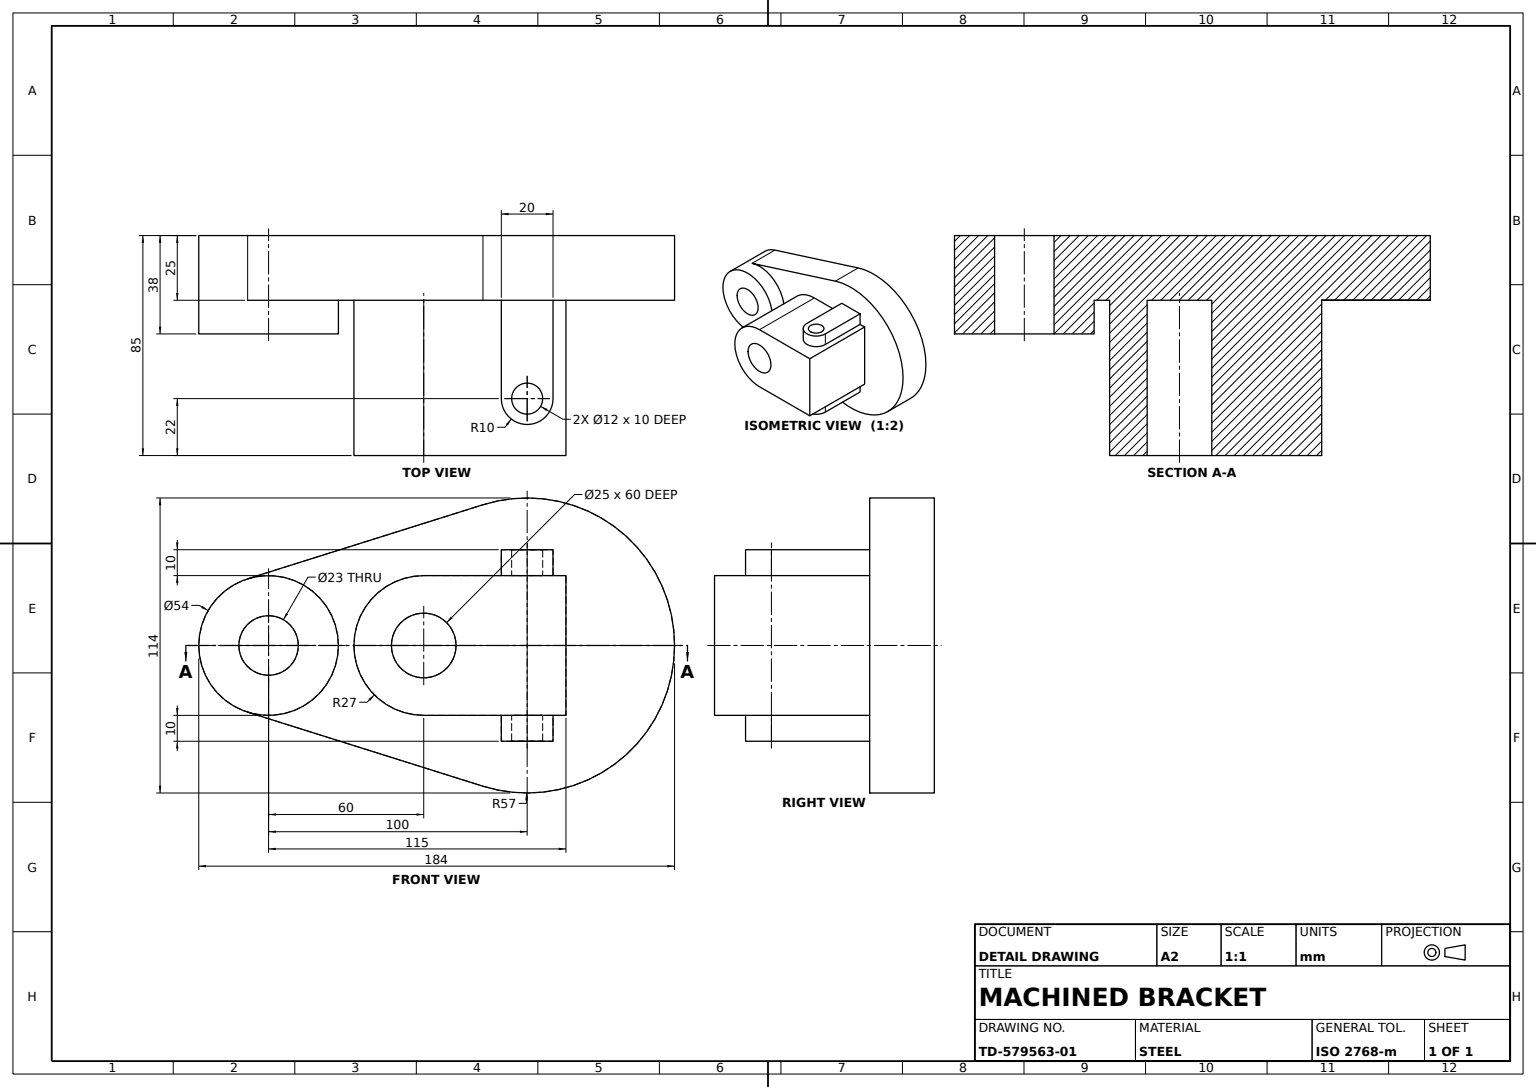
SolidWorks part; units mm, degrees
material "Plain Carbon Steel"
ref_plane "Front Plane" through (0, 0, 0) normal (0, 0, 1) x (1, 0, 0)
ref_plane "Top Plane" through (0, 0, 0) normal (0, 1, 0) x (1, 0, 0)
ref_plane "Right Plane" through (0, 0, 0) normal (1, 0, 0) x (0, 0, -1)
sketch "Pivot Boss Sketch" plane through (0, 0, 0) normal (0, 0, 1) x (1, 0, 0)
  circle A0 centre (0, 0) radius 11.5
  circle A1 centre (0, 0) radius 27
  dimension "D1" = 54
  dimension "D2" = 23
extrude "Pivot Boss" add sketch "Pivot Boss Sketch" along normal blind 38
ref_plane "Plane1" through (0, 0, 0) normal (0, 0, 1) x (1, 0, 0)
sketch "Mounting Plate Sketch" plane through (0, 0, 0) normal (0, 0, 1) x (1, 0, 0)
  line L0 (0, 0) -> (100, 0) construction
  line L1 (-8.1, 25.7564) -> (82.9, 54.3745)
  line L2 (-8.1, -25.7564) -> (82.9, -54.3745)
  arc A0 (82.9, -54.3745) -> (82.9, 54.3745) centre (100, 0) ccw
  circle A1 centre (0, 0) radius 27 construction
  arc A2 (-8.1, -25.7564) -> (-8.1, 25.7564) centre (0, 0) ccw
  dimension "D1" = 100
  dimension "D2" = 114
extrude "Mounting Plate" add sketch "Mounting Plate Sketch" along normal blind 25
sketch "Arm Block Sketch" plane through (0, 0, 25) normal (0, 0, 1) x (1, 0, 0)
  line L0 (0, 0) -> (100, 0) construction
  line L1 (100, 0) -> (60, 0) construction
  line L2 (60, 27) -> (115, 27)
  line L3 (115, 27) -> (115, -27)
  line L4 (115, -27) -> (60, -27)
  arc A0 (60, 27) -> (60, -27) centre (60, 0) ccw
  dimension "D1" = 27
  dimension "D2" = 115
  dimension "D3" = 60
extrude "Arm Block" add sketch "Arm Block Sketch" along normal blind 60
sketch "Pivot Bore Sketch" plane through (0, 0, 85) normal (0, 0, 1) x (1, 0, 0)
  circle A0 centre (60, 0) radius 12.5
  dimension "D1" = 25
extrude "Pivot Bore Ø25" cut sketch "Pivot Bore Sketch" against normal blind 60
sketch "Clamp Tab Sketch" plane through (0, -27, 0) normal (0, -1, 0) x (1, 0, 0)
  line L0 (157, 25) -> (82.9, 25) construction
  line L1 (115, 85) -> (115, 25) construction
  line L2 (90, 63) -> (90, 25)
  line L3 (60, 25) -> (115, 25) construction
  line L4 (90, 25) -> (110, 25)
  line L5 (110, 25) -> (110, 63)
  arc A0 (110, 63) -> (90, 63) centre (100, 63) ccw
  circle A1 centre (100, 63) radius 6
  dimension "D1" = 20
  dimension "D2" = 12
  dimension "D3" = 38
  dimension "D4" = 15
extrude "Clamp Tab" add sketch "Clamp Tab Sketch" along normal blind 10
ref_plane "Plane2" through (0, 0, 0) normal (0, 1, 0) x (1, 0, 0)
mirror "Clamp Tab Mirror" about plane through (0, 0, 0) normal (0, 1, 0) of "Clamp Tab"
